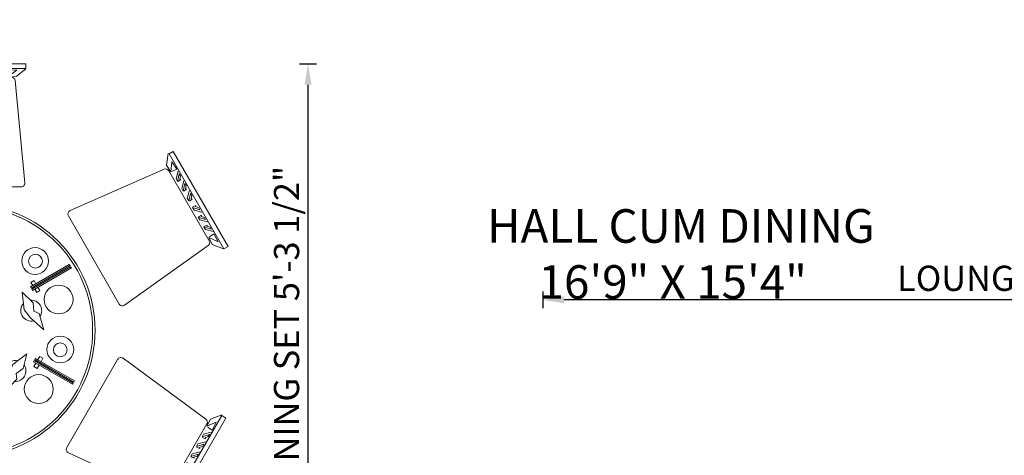
# Model space of a CAD drawing. Units: inches. Extents: x 1961 to 3038, y 800 to 1438.
# Tile 9 of 13: x 2803 to 2920, y 1096 to 1148. Entities that reach past the tile are written whole.
import ezdxf

# ---------------------------------------------------------------- set-up
doc = ezdxf.new("R2010")
doc.units = ezdxf.units.IN
for name, color, linetype, lineweight in [('A-ANNO-DIMS', 2, 'Continuous', 18), ('A-AREA-IDEN', 7, 'Continuous', 25), ('A-FURN', 8, 'Continuous', 18)]:
    doc.layers.add(name, color=color, linetype=linetype, lineweight=lineweight)
doc.styles.get("Standard").update_dxf_attribs({"font": 'arial.ttf'})
doc.dimstyles.new('ISO-25', dxfattribs={"dimtxt": 3, "dimasz": 2.5, "dimexe": 1, "dimexo": 1, "dimtad": 1, "dimdec": 4, "dimlunit": 4, "dimtxsty": 'Standard', "dimcen": 2.5, "dimadec": 0, "dimazin": 0, "dimtfac": 1, "dimtdec": 4, "dimtmove": 0, "dimatfit": 3, "dimfxl": 1, "dimfxlon": 1, "dimarcsym": 0})

# ---------------------------------------------------------------- blocks, each defined once
blk = doc.blocks.new('A$C1C317F9A')
for p, q in [((0.8788, 2.2685), (0.8788, 2.2478)), ((1.3449, 2.2685), (0.8788, 2.2685)), ((1.3449, 2.2478), (1.3449, 2.2685)), ((0.8756, 2.2462), (0.9155, 2.2143)), ((0.8788, 2.2478), (1.3449, 2.2478)), ((0.9139, 2.2414), (0.9522, 2.243)), ((0.949, 2.2159), (0.9139, 2.2414)), ((0.9522, 2.243), (0.9506, 2.2206)), ((0.9618, 2.2446), (0.9857, 2.2206)), ((0.9745, 2.243), (0.9841, 2.243)), ((0.9985, 2.2206), (0.9745, 2.243)), ((0.9841, 2.243), (0.9953, 2.2334)), ((0.9857, 2.2206), (0.9985, 2.2206)), ((0.9953, 2.2334), (0.9985, 2.2366)), ((0.9985, 2.2366), (1.0001, 2.2222)), ((1.0097, 2.2446), (1.0336, 2.2206)), ((1.0224, 2.243), (1.032, 2.243)), ((1.0464, 2.2206), (1.0224, 2.243)), ((1.032, 2.243), (1.0432, 2.2334)), ((1.0336, 2.2206), (1.0464, 2.2206)), ((1.0432, 2.2334), (1.0464, 2.2366)), ((1.0464, 2.2366), (1.048, 2.2222)), ((1.0576, 2.2446), (1.0815, 2.2206)), ((1.0703, 2.243), (1.0799, 2.243)), ((1.0943, 2.2206), (1.0703, 2.243)), ((1.0799, 2.243), (1.0911, 2.2334)), ((1.0815, 2.2206), (1.0943, 2.2206)), ((1.0911, 2.2334), (1.0943, 2.2366)), ((1.0943, 2.2366), (1.0959, 2.2222)), ((1.1262, 2.2366), (1.1246, 2.2222)), ((1.1262, 2.2206), (1.1502, 2.243)), ((1.1294, 2.2334), (1.1262, 2.2366)), ((1.139, 2.2206), (1.1262, 2.2206)), ((1.1406, 2.243), (1.1294, 2.2334)), ((1.1629, 2.2446), (1.139, 2.2206)), ((1.1502, 2.243), (1.1406, 2.243)), ((1.1741, 2.2366), (1.1725, 2.2222)), ((1.1741, 2.2206), (1.1981, 2.243)), ((1.1773, 2.2334), (1.1741, 2.2366)), ((1.1869, 2.2206), (1.1741, 2.2206)), ((1.1885, 2.243), (1.1773, 2.2334)), ((1.2108, 2.2446), (1.1869, 2.2206)), ((1.1981, 2.243), (1.1885, 2.243)), ((1.222, 2.2366), (1.2204, 2.2222)), ((1.222, 2.2206), (1.246, 2.243)), ((1.2252, 2.2334), (1.222, 2.2366)), ((1.2348, 2.2206), (1.222, 2.2206)), ((1.2364, 2.243), (1.2252, 2.2334)), ((1.2587, 2.2446), (1.2348, 2.2206)), ((1.246, 2.243), (1.2364, 2.243)), ((1.2683, 2.243), (1.2699, 2.2206)), ((1.3066, 2.2414), (1.2683, 2.243)), ((1.2715, 2.2159), (1.3066, 2.2414)), ((1.3449, 2.2462), (1.305, 2.2143)), ((0.8775, 1.7628), (0.9251, 2.1968)), ((0.9155, 2.2143), (0.949, 2.2159)), ((0.941, 2.2111), (1.2841, 2.2111)), ((1.305, 2.2143), (1.2715, 2.2159)), ((1.3, 2.1966), (1.3417, 1.7626)), ((0.2422, 1.9115), (0.0091, 1.5078)), ((0.0271, 1.4974), (0.2602, 1.9011)), ((0.2602, 1.9011), (0.2422, 1.9115)), ((0.2615, 1.9003), (0.2692, 1.8498)), ((1.9514, 1.8873), (1.9438, 1.8368)), ((1.9724, 1.8957), (1.9544, 1.8854)), ((1.9544, 1.8854), (2.1875, 1.4816)), ((2.2055, 1.492), (1.9724, 1.8957)), ((0.2465, 1.8648), (0.226, 1.8324)), ((0.2511, 1.8216), (0.2465, 1.8648)), ((0.2692, 1.8498), (0.2511, 1.8216)), ((1.9619, 1.8086), (1.9665, 1.8518)), ((1.9665, 1.8518), (1.987, 1.8194)), ((0.09, 1.5329), (0.2615, 1.8301)), ((0.2148, 1.813), (0.21, 1.8047)), ((0.21, 1.8047), (0.2127, 1.7903)), ((0.2222, 1.7811), (0.2148, 1.813)), ((0.2198, 1.8249), (0.2286, 1.7922)), ((0.226, 1.8324), (0.2461, 1.8226)), ((0.282, 1.8367), (0.6787, 1.6557)), ((1.5338, 1.644), (1.9335, 1.8198)), ((1.9438, 1.8368), (1.9619, 1.8086)), ((1.9537, 1.8131), (2.1253, 1.516)), ((1.987, 1.8194), (1.9669, 1.8096)), ((1.9932, 1.8119), (1.9844, 1.7792)), ((0.1909, 1.7716), (0.1861, 1.7633)), ((0.1861, 1.7633), (0.1888, 1.7488)), ((0.1982, 1.7396), (0.1909, 1.7716)), ((0.1959, 1.7834), (0.2046, 1.7507)), ((0.2127, 1.7903), (0.2084, 1.7891)), ((0.2084, 1.7891), (0.22, 1.7805)), ((0.2286, 1.7922), (0.2222, 1.7811)), ((1.9844, 1.7792), (1.9908, 1.7681)), ((1.9908, 1.7681), (1.9982, 1.8)), ((2.0046, 1.7761), (1.993, 1.7675)), ((1.9982, 1.8), (2.003, 1.7917)), ((2.003, 1.7917), (2.0003, 1.7773)), ((2.0003, 1.7773), (2.0046, 1.7761)), ((2.0171, 1.7704), (2.0084, 1.7377)), ((0.1669, 1.7301), (0.1621, 1.7218)), ((0.1621, 1.7218), (0.1648, 1.7073)), ((0.1743, 1.6982), (0.1669, 1.7301)), ((0.1719, 1.7419), (0.1807, 1.7092)), ((0.1888, 1.7488), (0.1844, 1.7476)), ((0.1844, 1.7476), (0.1961, 1.7391)), ((0.2046, 1.7507), (0.1982, 1.7396)), ((1.3258, 1.7451), (0.8934, 1.7451)), ((2.0084, 1.7377), (2.0147, 1.7266)), ((2.0147, 1.7266), (2.0221, 1.7585)), ((2.0286, 1.7346), (2.0169, 1.726)), ((2.0221, 1.7585), (2.0269, 1.7502)), ((2.0269, 1.7502), (2.0242, 1.7358)), ((2.0242, 1.7358), (2.0286, 1.7346)), ((2.0411, 1.7289), (2.0323, 1.6962)), ((2.0387, 1.6852), (2.0461, 1.7171)), ((2.0461, 1.7171), (2.0509, 1.7088)), ((0.1445, 1.6785), (0.1577, 1.6727)), ((0.1457, 1.6741), (0.1445, 1.6785)), ((0.1648, 1.7073), (0.1605, 1.7061)), ((0.1605, 1.7061), (0.1721, 1.6976)), ((0.1807, 1.7092), (0.1743, 1.6982)), ((2.0323, 1.6962), (2.0387, 1.6852)), ((2.0525, 1.6931), (2.0409, 1.6846)), ((2.0509, 1.7088), (2.0482, 1.6943)), ((2.0482, 1.6943), (2.0525, 1.6931)), ((0.1192, 1.6507), (0.1519, 1.6595)), ((0.1217, 1.6327), (0.1206, 1.637)), ((0.1206, 1.637), (0.1338, 1.6312)), ((0.1583, 1.6705), (0.127, 1.6609)), ((0.127, 1.6609), (0.1318, 1.6692)), ((0.1318, 1.6692), (0.1457, 1.6741)), ((0.1519, 1.6595), (0.1583, 1.6705)), ((0.6859, 1.6332), (0.4697, 1.2588)), ((1.091, 1.6437, 0.0908), (1.091, 1.4528, 0.0908)), ((1.097, 1.6437, 0.0908), (1.091, 1.6437, 0.0908)), ((1.097, 1.4528, 0.0908), (1.097, 1.6437, 0.0908)), ((1.1023, 1.6437, 0.0908), (1.1023, 1.4528, 0.0908)), ((1.1083, 1.6437, 0.0908), (1.1023, 1.6437, 0.0908)), ((1.1083, 1.4528, 0.0908), (1.1083, 1.6437, 0.0908)), ((2.0547, 1.6575), (2.086, 1.6479)), ((2.061, 1.6464), (2.0547, 1.6575)), ((2.0685, 1.6655), (2.0552, 1.6597)), ((2.0937, 1.6377), (2.061, 1.6464)), ((2.0673, 1.6611), (2.0685, 1.6655)), ((2.0812, 1.6562), (2.0673, 1.6611)), ((2.086, 1.6479), (2.0812, 1.6562)), ((0.0839, 1.5863), (0.0978, 1.5912)), ((0.0953, 1.6092), (0.128, 1.618)), ((0.0966, 1.5955), (0.1098, 1.5897)), ((0.0978, 1.5912), (0.0966, 1.5955)), ((0.1344, 1.629), (0.1031, 1.6195)), ((0.1031, 1.6195), (0.1078, 1.6278)), ((0.1078, 1.6278), (0.1217, 1.6327)), ((0.128, 1.618), (0.1344, 1.629)), ((1.7426, 1.2469), (1.5264, 1.6214)), ((2.0786, 1.616), (2.1099, 1.6065)), ((2.085, 1.605), (2.0786, 1.616)), ((2.0924, 1.624), (2.0792, 1.6182)), ((2.1177, 1.5962), (2.085, 1.605)), ((2.0913, 1.6196), (2.0924, 1.624)), ((2.1051, 1.6148), (2.0913, 1.6196)), ((2.1099, 1.6065), (2.1051, 1.6148)), ((0.0502, 1.5246), (0.0679, 1.5586)), ((0.0679, 1.5586), (0.0865, 1.5461)), ((0.0713, 1.5677), (0.104, 1.5765)), ((0.1104, 1.5876), (0.0791, 1.578)), ((0.0791, 1.578), (0.0839, 1.5863)), ((0.104, 1.5765), (0.1104, 1.5876)), ((2.1026, 1.5745), (2.1339, 1.565)), ((2.1089, 1.5635), (2.1026, 1.5745)), ((2.1164, 1.5825), (2.1031, 1.5767)), ((2.1416, 1.5547), (2.1089, 1.5635)), ((2.1152, 1.5782), (2.1164, 1.5825)), ((2.1291, 1.5733), (2.1152, 1.5782)), ((2.1339, 1.565), (2.1291, 1.5733)), ((0.0091, 1.5078), (0.0271, 1.4974)), ((0.0269, 1.4939), (0.0745, 1.5125)), ((0.0898, 1.5423), (0.0502, 1.5246)), ((0.0745, 1.5125), (0.0898, 1.5423)), ((0.4464, 1.2539), (0.0943, 1.5121)), ((2.1232, 1.5293), (2.1628, 1.5116)), ((2.1385, 1.4995), (2.1232, 1.5293)), ((2.145, 1.5456), (2.1265, 1.5331)), ((2.1628, 1.5116), (2.145, 1.5456)), ((1.0755, 1.4796, 0.0908), (1.0755, 1.4641, 0.0908)), ((1.091, 1.4796, 0.0908), (1.0755, 1.4796, 0.0908)), ((1.1023, 1.4796, 0.0908), (1.097, 1.4796, 0.0908)), ((1.125, 1.4796, 0.0908), (1.1083, 1.4796, 0.0908)), ((1.125, 1.4641, 0.0908), (1.125, 1.4796, 0.0908)), ((2.1208, 1.495), (1.7657, 1.2419)), ((2.1861, 1.4809), (2.1385, 1.4995)), ((2.1875, 1.4816), (2.2055, 1.492)), ((1.0755, 1.4641, 0.0908), (1.091, 1.4641, 0.0908)), ((1.091, 1.4528, 0.0908), (1.097, 1.4528, 0.0908)), ((1.1549, 1.429, 0.0908), (1.0933, 1.4112, 0.0908)), ((1.097, 1.4641, 0.0908), (1.1023, 1.4641, 0.0908)), ((1.1023, 1.4528, 0.0908), (1.1083, 1.4528, 0.0908)), ((1.1083, 1.4641, 0.0908), (1.125, 1.4641, 0.0908)), ((1.1882, 1.4134, 0.0908), (1.1549, 1.429, 0.0908)), ((1.2075, 1.4282, 0.0908), (1.1882, 1.4134, 0.0908)), ((1.278, 1.4112, 0.0908), (1.2075, 1.4282, 0.0908)), ((0.6765, 1.3825, 0.0908), (0.6735, 1.3774, 0.0908)), ((0.8419, 1.2871, 0.0908), (0.6765, 1.3825, 0.0908)), ((0.6822, 1.3924, 0.0908), (0.6792, 1.3872, 0.0908)), ((0.6792, 1.3872, 0.0908), (0.8446, 1.2917, 0.0908)), ((0.8476, 1.2969, 0.0908), (0.6822, 1.3924, 0.0908)), ((0.9684, 1.4231, 0.0908), (0.9184, 1.3706, 0.0908)), ((0.953, 1.3489, 0.0908), (0.9684, 1.4231, 0.0908)), ((1.0933, 1.4112, 0.0908), (1.1623, 1.3815, 0.0908)), ((1.1623, 1.3815, 0.0908), (1.2061, 1.3874, 0.0908)), ((1.2061, 1.3874, 0.0908), (1.278, 1.4112, 0.0908)), ((1.5304, 1.4154, 0.0908), (1.365, 1.3199, 0.0908)), ((1.368, 1.3147, 0.0908), (1.5334, 1.4102, 0.0908)), ((1.5361, 1.4055, 0.0908), (1.3707, 1.3101, 0.0908)), ((1.3737, 1.3049, 0.0908), (1.539, 1.4004, 0.0908)), ((1.5334, 1.4102, 0.0908), (1.5304, 1.4154, 0.0908)), ((1.539, 1.4004, 0.0908), (1.5361, 1.4055, 0.0908)), ((0.6735, 1.3774, 0.0908), (0.8389, 1.2819, 0.0908)), ((0.9216, 1.3464, 0.0908), (0.8914, 1.3253, 0.0908)), ((0.9184, 1.3706, 0.0908), (0.9216, 1.3464, 0.0908)), ((0.9363, 1.308, 0.0908), (0.953, 1.3489, 0.0908)), ((1.3805, 1.3467, 0.0908), (1.3671, 1.339, 0.0908)), ((1.3883, 1.3333, 0.0908), (1.3805, 1.3467, 0.0908)), ((0.8213, 1.3051, 0.0908), (0.8186, 1.3005, 0.0908)), ((0.8327, 1.3248, 0.0908), (0.8243, 1.3103, 0.0908)), ((0.8461, 1.317, 0.0908), (0.8327, 1.3248, 0.0908)), ((0.8377, 1.3025, 0.0908), (0.8461, 1.317, 0.0908)), ((0.8914, 1.3253, 0.0908), (0.8761, 1.2631, 0.0908)), ((0.8761, 1.2631, 0.0908), (0.9363, 1.308, 0.0908)), ((1.365, 1.3199, 0.0908), (1.368, 1.3147, 0.0908)), ((1.3671, 1.339, 0.0908), (1.3748, 1.3255, 0.0908)), ((1.3707, 1.3101, 0.0908), (1.3737, 1.3049, 0.0908)), ((1.3778, 1.3204, 0.0908), (1.3805, 1.3157, 0.0908)), ((1.3835, 1.3106, 0.0908), (1.3918, 1.2961, 0.0908)), ((1.3939, 1.3235, 0.0908), (1.3912, 1.3281, 0.0908)), ((1.3918, 1.2961, 0.0908), (1.4053, 1.3038, 0.0908)), ((1.4053, 1.3038, 0.0908), (1.3969, 1.3183, 0.0908)), ((0.8156, 1.2953, 0.0908), (0.8079, 1.2819, 0.0908)), ((0.8079, 1.2819, 0.0908), (0.8213, 1.2741, 0.0908)), ((0.8213, 1.2741, 0.0908), (0.8291, 1.2876, 0.0908)), ((0.8321, 1.2927, 0.0908), (0.8348, 1.2974, 0.0908)), ((0.8389, 1.2819, 0.0908), (0.8419, 1.2871, 0.0908)), ((0.8446, 1.2917, 0.0908), (0.8476, 1.2969, 0.0908)), ((1.3763, 1.2527, 0.0908), (1.3301, 1.2971, 0.0908)), ((1.3301, 1.2971, 0.0908), (1.3389, 1.2225, 0.0908)), ((1.3389, 1.2225, 0.0908), (1.366, 1.1876, 0.0908)), ((1.3795, 1.216, 0.0908), (1.3763, 1.2527, 0.0908)), ((1.402, 1.2067, 0.0908), (1.3795, 1.216, 0.0908)), ((1.366, 1.1876, 0.0908), (1.4225, 1.1371, 0.0908)), ((1.4225, 1.1371, 0.0908), (1.402, 1.2067, 0.0908)), ((0.8033, 1.1609, 0.0908), (0.8238, 1.0913, 0.0908)), ((0.8599, 1.1105, 0.0908), (0.8033, 1.1609, 0.0908)), ((0.8238, 1.0913, 0.0908), (0.8463, 1.0821, 0.0908)), ((0.8869, 1.0755, 0.0908), (0.8599, 1.1105, 0.0908)), ((0.8463, 1.0821, 0.0908), (0.8495, 1.0454, 0.0908)), ((0.8957, 1.0009, 0.0908), (0.8869, 1.0755, 0.0908)), ((0.0847, 0.7751), (0.4398, 1.0281)), ((0.4628, 1.0231), (0.679, 0.6486)), ((0.8495, 1.0454, 0.0908), (0.8957, 1.0009, 0.0908)), ((1.3498, 1.0349, 0.0908), (1.2896, 0.99, 0.0908)), ((1.3344, 0.9727, 0.0908), (1.3498, 1.0349, 0.0908)), ((1.3813, 1.0063, 0.0908), (1.3783, 1.0011, 0.0908)), ((1.5466, 0.9108, 0.0908), (1.3813, 1.0063, 0.0908)), ((1.3869, 1.0161, 0.0908), (1.384, 1.011, 0.0908)), ((1.384, 1.011, 0.0908), (1.5493, 0.9155, 0.0908)), ((1.5523, 0.9207, 0.0908), (1.3869, 1.0161, 0.0908)), ((1.3938, 1.0053, 0.0908), (1.3911, 1.0006, 0.0908)), ((1.4045, 1.0239, 0.0908), (1.3968, 1.0105, 0.0908)), ((1.418, 1.0162, 0.0908), (1.4045, 1.0239, 0.0908)), ((1.4102, 1.0027, 0.0908), (1.418, 1.0162, 0.0908)), ((1.5196, 0.6368), (1.7358, 1.0113)), ((1.7591, 1.0162), (2.1111, 0.7579)), ((0.8522, 0.9931, 0.0908), (0.6868, 0.8977, 0.0908)), ((0.6898, 0.8925, 0.0908), (0.8552, 0.988, 0.0908)), ((0.8578, 0.9833, 0.0908), (0.6925, 0.8878, 0.0908)), ((0.6955, 0.8827, 0.0908), (0.8608, 0.9781, 0.0908)), ((0.834, 1.0019, 0.0908), (0.8206, 0.9942, 0.0908)), ((0.8206, 0.9942, 0.0908), (0.8289, 0.9797, 0.0908)), ((0.8319, 0.9745, 0.0908), (0.8346, 0.9699, 0.0908)), ((0.8424, 0.9875, 0.0908), (0.834, 1.0019, 0.0908)), ((0.8376, 0.9647, 0.0908), (0.8453, 0.9513, 0.0908)), ((0.848, 0.9776, 0.0908), (0.8453, 0.9823, 0.0908)), ((0.8588, 0.959, 0.0908), (0.851, 0.9725, 0.0908)), ((0.8552, 0.988, 0.0908), (0.8522, 0.9931, 0.0908)), ((0.8608, 0.9781, 0.0908), (0.8578, 0.9833, 0.0908)), ((1.2896, 0.99, 0.0908), (1.2728, 0.9491, 0.0908)), ((1.3042, 0.9516, 0.0908), (1.3344, 0.9727, 0.0908)), ((1.3783, 1.0011, 0.0908), (1.5437, 0.9057, 0.0908)), ((1.3881, 0.9955, 0.0908), (1.3797, 0.981, 0.0908)), ((1.3797, 0.981, 0.0908), (1.3932, 0.9732, 0.0908)), ((1.3932, 0.9732, 0.0908), (1.4015, 0.9877, 0.0908)), ((1.4045, 0.9929, 0.0908), (1.4072, 0.9975, 0.0908)), ((0.8453, 0.9513, 0.0908), (0.8588, 0.959, 0.0908)), ((1.2728, 0.9491, 0.0908), (1.2574, 0.875, 0.0908)), ((1.2574, 0.875, 0.0908), (1.3074, 0.9275, 0.0908)), ((1.3074, 0.9275, 0.0908), (1.3042, 0.9516, 0.0908)), ((0.6868, 0.8977, 0.0908), (0.6898, 0.8925, 0.0908)), ((0.6925, 0.8878, 0.0908), (0.6955, 0.8827, 0.0908)), ((1.0198, 0.9106, 0.0908), (0.9478, 0.8869, 0.0908)), ((0.9478, 0.8869, 0.0908), (1.0183, 0.8698, 0.0908)), ((1.0183, 0.8698, 0.0908), (1.0376, 0.8846, 0.0908)), ((1.0636, 0.9165, 0.0908), (1.0198, 0.9106, 0.0908)), ((1.0376, 0.8846, 0.0908), (1.071, 0.8691, 0.0908)), ((1.1326, 0.8869, 0.0908), (1.0636, 0.9165, 0.0908)), ((1.071, 0.8691, 0.0908), (1.1326, 0.8869, 0.0908)), ((1.5437, 0.9057, 0.0908), (1.5466, 0.9108, 0.0908)), ((1.5493, 0.9155, 0.0908), (1.5523, 0.9207, 0.0908)), ((1.1235, 0.8453, 0.0908), (1.1175, 0.8453, 0.0908)), ((1.1175, 0.8453, 0.0908), (1.1175, 0.6543, 0.0908)), ((1.1235, 0.6543, 0.0908), (1.1235, 0.8453, 0.0908)), ((1.1349, 0.8453, 0.0908), (1.1289, 0.8453, 0.0908)), ((1.1289, 0.8453, 0.0908), (1.1289, 0.6543, 0.0908)), ((1.1349, 0.6543, 0.0908), (1.1349, 0.8453, 0.0908)), ((1.1175, 0.8339, 0.0908), (1.1008, 0.8339, 0.0908)), ((1.1008, 0.8339, 0.0908), (1.1008, 0.8184, 0.0908)), ((1.1008, 0.8184, 0.0908), (1.1175, 0.8184, 0.0908)), ((1.1289, 0.8339, 0.0908), (1.1235, 0.8339, 0.0908)), ((1.1235, 0.8184, 0.0908), (1.1289, 0.8184, 0.0908)), ((1.1504, 0.8339, 0.0908), (1.1349, 0.8339, 0.0908)), ((1.1349, 0.8184, 0.0908), (1.1504, 0.8184, 0.0908)), ((1.1504, 0.8184, 0.0908), (1.1504, 0.8339, 0.0908)), ((0.018, 0.7884), (0, 0.778)), ((0, 0.778), (0.2331, 0.3743)), ((0.2511, 0.3847), (0.018, 0.7884)), ((0.0193, 0.7892), (0.0669, 0.7706)), ((0.0427, 0.7584), (0.0604, 0.7244)), ((0.0823, 0.7407), (0.0427, 0.7584)), ((0.0669, 0.7706), (0.0823, 0.7407)), ((0.2517, 0.4569), (0.0802, 0.7541)), ((2.1784, 0.7726), (1.9453, 0.3689)), ((1.9633, 0.3585), (2.1964, 0.7622)), ((2.131, 0.7576), (2.1156, 0.7277)), ((2.1786, 0.7762), (2.131, 0.7576)), ((2.1964, 0.7622), (2.1784, 0.7726)), ((0.0604, 0.7244), (0.079, 0.737)), ((0.0638, 0.7153), (0.0965, 0.7066)), ((2.1155, 0.7371), (1.9439, 0.4399)), ((2.1156, 0.7277), (2.1553, 0.7454)), ((2.1375, 0.7114), (2.119, 0.724)), ((2.1553, 0.7454), (2.1375, 0.7114)), ((0.0716, 0.7051), (0.0764, 0.6968)), ((0.1029, 0.6955), (0.0716, 0.7051)), ((0.0764, 0.6968), (0.0903, 0.6919)), ((0.0878, 0.6738), (0.1205, 0.6651)), ((0.0891, 0.6875), (0.1023, 0.6933)), ((0.0903, 0.6919), (0.0891, 0.6875)), ((0.0965, 0.7066), (0.1029, 0.6955)), ((2.1014, 0.6935), (2.095, 0.6825)), ((2.095, 0.6825), (2.1264, 0.6921)), ((2.1089, 0.6745), (2.0956, 0.6803)), ((2.1341, 0.7023), (2.1014, 0.6935)), ((2.1216, 0.6838), (2.1077, 0.6789)), ((2.1077, 0.6789), (2.1089, 0.6745)), ((2.1264, 0.6921), (2.1216, 0.6838)), ((0.0955, 0.6636), (0.1003, 0.6553)), ((0.1269, 0.654), (0.0955, 0.6636)), ((0.1003, 0.6553), (0.1142, 0.6504)), ((0.1117, 0.6324), (0.1444, 0.6236)), ((0.1131, 0.646), (0.1263, 0.6518)), ((0.1142, 0.6504), (0.1131, 0.646)), ((0.1205, 0.6651), (0.1269, 0.654)), ((1.1175, 0.6543, 0.0908), (1.1235, 0.6543, 0.0908)), ((1.1289, 0.6543, 0.0908), (1.1349, 0.6543, 0.0908)), ((2.0775, 0.6521), (2.0711, 0.641)), ((2.0711, 0.641), (2.1024, 0.6506)), ((2.0849, 0.633), (2.0717, 0.6388)), ((2.1102, 0.6608), (2.0775, 0.6521)), ((2.0976, 0.6423), (2.0837, 0.6374)), ((2.0837, 0.6374), (2.0849, 0.633)), ((2.1024, 0.6506), (2.0976, 0.6423)), ((0.1195, 0.6221), (0.1243, 0.6138)), ((0.1508, 0.6125), (0.1195, 0.6221)), ((0.1243, 0.6138), (0.1382, 0.6089)), ((0.137, 0.6046), (0.1502, 0.6104)), ((0.1382, 0.6089), (0.137, 0.6046)), ((0.1444, 0.6236), (0.1508, 0.6125)), ((0.6716, 0.6261), (0.272, 0.4503)), ((1.9235, 0.4334), (1.5268, 0.6143)), ((2.0535, 0.6106), (2.0471, 0.5995)), ((2.0471, 0.5995), (2.0785, 0.6091)), ((2.061, 0.5915), (2.0477, 0.5973)), ((2.0862, 0.6194), (2.0535, 0.6106)), ((2.0737, 0.6008), (2.0598, 0.5959)), ((2.0598, 0.5959), (2.061, 0.5915)), ((2.0785, 0.6091), (2.0737, 0.6008)), ((0.153, 0.5769), (0.1646, 0.5855)), ((0.1573, 0.5757), (0.153, 0.5769)), ((0.1546, 0.5613), (0.1573, 0.5757)), ((0.1594, 0.553), (0.1546, 0.5613)), ((0.1668, 0.5849), (0.1594, 0.553)), ((0.1644, 0.5411), (0.1732, 0.5738)), ((0.1732, 0.5738), (0.1668, 0.5849)), ((2.0248, 0.5608), (2.0312, 0.5719)), ((2.0336, 0.5281), (2.0248, 0.5608)), ((2.0312, 0.5719), (2.0386, 0.54)), ((2.045, 0.5639), (2.0334, 0.5725)), ((2.0386, 0.54), (2.0433, 0.5483)), ((2.0406, 0.5627), (2.045, 0.5639)), ((2.0433, 0.5483), (2.0406, 0.5627)), ((0.1769, 0.5354), (0.1885, 0.544)), ((0.1813, 0.5343), (0.1769, 0.5354)), ((0.1786, 0.5198), (0.1813, 0.5343)), ((0.1834, 0.5115), (0.1786, 0.5198)), ((0.1907, 0.5434), (0.1834, 0.5115)), ((0.1884, 0.4996), (0.1971, 0.5323)), ((0.1971, 0.5323), (0.1907, 0.5434)), ((0.2009, 0.4939), (0.2125, 0.5025)), ((0.9055, 0.0734), (0.8638, 0.5074)), ((0.9096, 0.0719), (0.8679, 0.5059)), ((0.8797, 0.5249), (1.3121, 0.5249)), ((0.8838, 0.5234), (1.3162, 0.5234)), ((1.328, 0.5072), (1.2804, 0.0732)), ((1.3321, 0.5057), (1.2845, 0.0717)), ((2.0009, 0.5193), (2.0072, 0.5304)), ((2.0096, 0.4866), (2.0009, 0.5193)), ((2.0072, 0.5304), (2.0146, 0.4985)), ((2.0211, 0.5224), (2.0094, 0.531)), ((2.0146, 0.4985), (2.0194, 0.5068)), ((2.0167, 0.5212), (2.0211, 0.5224)), ((2.0194, 0.5068), (2.0167, 0.5212)), ((0.2052, 0.4928), (0.2009, 0.4939)), ((0.2025, 0.4783), (0.2052, 0.4928)), ((0.2073, 0.47), (0.2025, 0.4783)), ((0.2147, 0.5019), (0.2073, 0.47)), ((0.2123, 0.4582), (0.2211, 0.4909)), ((0.2211, 0.4909), (0.2147, 0.5019)), ((0.2436, 0.4615), (0.239, 0.4183)), ((0.2617, 0.4332), (0.2436, 0.4615)), ((1.9769, 0.4779), (1.9833, 0.4889)), ((1.9857, 0.4451), (1.9769, 0.4779)), ((1.9833, 0.4889), (1.9907, 0.457)), ((1.9971, 0.4809), (1.9855, 0.4895)), ((1.9907, 0.457), (1.9955, 0.4653)), ((1.9927, 0.4798), (1.9971, 0.4809)), ((1.9955, 0.4653), (1.9927, 0.4798)), ((0.2185, 0.4507), (0.2386, 0.4604)), ((0.239, 0.4183), (0.2185, 0.4507)), ((0.254, 0.3827), (0.2617, 0.4332)), ((1.9363, 0.4202), (1.9544, 0.4484)), ((1.9439, 0.3697), (1.9363, 0.4202)), ((1.9544, 0.4484), (1.9589, 0.4053)), ((1.9589, 0.4053), (1.9795, 0.4377)), ((1.9795, 0.4377), (1.9593, 0.4474)), ((0.2331, 0.3743), (0.2511, 0.3847)), ((1.9453, 0.3689), (1.9633, 0.3585)), ((0.8605, 0.0239), (0.9005, 0.0558)), ((0.8647, 0.0223), (0.9046, 0.0543)), ((0.934, 0.0542), (0.8989, 0.0286)), ((0.9005, 0.0558), (0.934, 0.0542)), ((0.9381, 0.0527), (0.903, 0.0271)), ((0.9046, 0.0543), (0.9381, 0.0527)), ((1.2645, 0.059), (0.9213, 0.059)), ((1.2686, 0.0574), (0.9255, 0.0574)), ((0.9372, 0.027), (0.9356, 0.0494)), ((0.9413, 0.0255), (0.9397, 0.0479)), ((0.9468, 0.0255), (0.9707, 0.0494)), ((0.9509, 0.0239), (0.9748, 0.0479)), ((0.9835, 0.0494), (0.9595, 0.027)), ((0.9876, 0.0479), (0.9636, 0.0255)), ((0.9707, 0.0494), (0.9835, 0.0494)), ((0.9748, 0.0479), (0.9876, 0.0479)), ((0.9835, 0.0334), (0.9851, 0.0478)), ((0.9876, 0.0319), (0.9892, 0.0463)), ((0.9946, 0.0255), (1.0186, 0.0494)), ((0.9988, 0.0239), (1.0227, 0.0479)), ((1.0314, 0.0494), (1.0074, 0.027)), ((1.0355, 0.0479), (1.0115, 0.0255)), ((1.0186, 0.0494), (1.0314, 0.0494)), ((1.0227, 0.0479), (1.0355, 0.0479)), ((1.0314, 0.0334), (1.033, 0.0478)), ((1.0355, 0.0319), (1.0371, 0.0463)), ((1.0425, 0.0255), (1.0665, 0.0494)), ((1.0467, 0.0239), (1.0706, 0.0479)), ((1.0793, 0.0494), (1.0553, 0.027)), ((1.0834, 0.0479), (1.0594, 0.0255)), ((1.0665, 0.0494), (1.0793, 0.0494)), ((1.0706, 0.0479), (1.0834, 0.0479)), ((1.0793, 0.0334), (1.0809, 0.0478)), ((1.0834, 0.0319), (1.085, 0.0463)), ((1.1112, 0.0334), (1.1096, 0.0478)), ((1.1112, 0.0494), (1.1351, 0.027)), ((1.124, 0.0494), (1.1112, 0.0494)), ((1.1153, 0.0319), (1.1137, 0.0463)), ((1.1153, 0.0479), (1.1393, 0.0255)), ((1.1281, 0.0479), (1.1153, 0.0479)), ((1.1479, 0.0255), (1.124, 0.0494)), ((1.152, 0.0239), (1.1281, 0.0479)), ((1.1591, 0.0334), (1.1575, 0.0478)), ((1.1591, 0.0494), (1.183, 0.027)), ((1.1719, 0.0494), (1.1591, 0.0494)), ((1.1632, 0.0319), (1.1616, 0.0463)), ((1.1632, 0.0479), (1.1872, 0.0255)), ((1.176, 0.0479), (1.1632, 0.0479)), ((1.1958, 0.0255), (1.1719, 0.0494)), ((1.1999, 0.0239), (1.176, 0.0479)), ((1.207, 0.0334), (1.2054, 0.0478)), ((1.207, 0.0494), (1.2309, 0.027)), ((1.2198, 0.0494), (1.207, 0.0494)), ((1.2111, 0.0319), (1.2095, 0.0463)), ((1.2111, 0.0479), (1.235, 0.0255)), ((1.2239, 0.0479), (1.2111, 0.0479)), ((1.2437, 0.0255), (1.2198, 0.0494)), ((1.2478, 0.0239), (1.2239, 0.0479)), ((1.2533, 0.027), (1.2549, 0.0494)), ((1.29, 0.0558), (1.2565, 0.0542)), ((1.2565, 0.0542), (1.2916, 0.0286)), ((1.2574, 0.0255), (1.259, 0.0479)), ((1.2941, 0.0543), (1.2606, 0.0527)), ((1.2606, 0.0527), (1.2957, 0.0271)), ((1.3299, 0.0239), (1.29, 0.0558)), ((1.334, 0.0223), (1.2941, 0.0543)), ((0.8605, 0.0223), (0.8605, 0.0015)), ((1.3267, 0.0223), (0.8605, 0.0223)), ((0.8605, 0.0015), (1.3267, 0.0015)), ((0.8647, 0.0207), (0.8647, 0)), ((1.3308, 0.0207), (0.8647, 0.0207)), ((0.8647, 0), (1.3308, 0)), ((0.8989, 0.0286), (0.9372, 0.027)), ((0.903, 0.0271), (0.9413, 0.0255)), ((0.9595, 0.027), (0.9691, 0.027)), ((0.9636, 0.0255), (0.9732, 0.0255)), ((0.9691, 0.027), (0.9803, 0.0366)), ((0.9732, 0.0255), (0.9844, 0.0351)), ((0.9803, 0.0366), (0.9835, 0.0334)), ((0.9844, 0.0351), (0.9876, 0.0319)), ((1.0074, 0.027), (1.017, 0.027)), ((1.0115, 0.0255), (1.0211, 0.0255)), ((1.017, 0.027), (1.0282, 0.0366)), ((1.0211, 0.0255), (1.0323, 0.0351)), ((1.0282, 0.0366), (1.0314, 0.0334)), ((1.0323, 0.0351), (1.0355, 0.0319)), ((1.0553, 0.027), (1.0649, 0.027)), ((1.0594, 0.0255), (1.069, 0.0255)), ((1.0649, 0.027), (1.0761, 0.0366)), ((1.069, 0.0255), (1.0802, 0.0351)), ((1.0761, 0.0366), (1.0793, 0.0334)), ((1.0802, 0.0351), (1.0834, 0.0319)), ((1.1144, 0.0366), (1.1112, 0.0334)), ((1.1256, 0.027), (1.1144, 0.0366)), ((1.1185, 0.0351), (1.1153, 0.0319)), ((1.1297, 0.0255), (1.1185, 0.0351)), ((1.1351, 0.027), (1.1256, 0.027)), ((1.1393, 0.0255), (1.1297, 0.0255)), ((1.1623, 0.0366), (1.1591, 0.0334)), ((1.1735, 0.027), (1.1623, 0.0366)), ((1.1664, 0.0351), (1.1632, 0.0319)), ((1.1776, 0.0255), (1.1664, 0.0351)), ((1.183, 0.027), (1.1735, 0.027)), ((1.1872, 0.0255), (1.1776, 0.0255)), ((1.2102, 0.0366), (1.207, 0.0334)), ((1.2214, 0.027), (1.2102, 0.0366)), ((1.2143, 0.0351), (1.2111, 0.0319)), ((1.2255, 0.0255), (1.2143, 0.0351)), ((1.2309, 0.027), (1.2214, 0.027)), ((1.235, 0.0255), (1.2255, 0.0255)), ((1.2916, 0.0286), (1.2533, 0.027)), ((1.2957, 0.0271), (1.2574, 0.0255)), ((1.3267, 0.0015), (1.3267, 0.0223)), ((1.3308, 0), (1.3308, 0.0207))]:
    blk.add_line(p, q)
for centre, radius in [((1.1027, 1.135), 0.537), ((1.1027, 1.135), 0.527), ((1.0059, 1.525, 0.0908), 0.0569), ((1.0072, 1.5257, 0.0908), 0.0294), ((1.1975, 1.5297, 0.0908), 0.0613), ((0.8256, 1.4126, 0.0908), 0.0613), ((1.385, 1.4297, 0.0908), 0.0569), ((1.3863, 1.4289, 0.0908), 0.0294), ((0.7338, 1.2443, 0.0908), 0.0569), ((1.4849, 1.2661, 0.0908), 0.0613), ((0.7339, 1.2458, 0.0908), 0.0294), ((0.741, 1.0319, 0.0908), 0.0613), ((1.4921, 1.0537, 0.0908), 0.0569), ((1.492, 1.0522, 0.0908), 0.0294), ((0.8408, 0.8683, 0.0908), 0.0569), ((1.4003, 0.8854, 0.0908), 0.0613), ((0.8396, 0.8691, 0.0908), 0.0294), ((1.0283, 0.7683, 0.0908), 0.0613), ((1.2199, 0.773, 0.0908), 0.0569), ((1.2186, 0.7723, 0.0908), 0.0294)]:
    blk.add_circle(centre, radius)
for centre, radius, start, end in [((0.941, 2.1951), 0.016, 90, 173.7428), ((1.2841, 2.1951), 0.016, 5.4801, 90), ((0.2754, 1.8222), 0.016, 65.4801, 150), ((1.9399, 1.8052), 0.016, 30, 113.7428), ((0.8934, 1.7611), 0.016, 173.7428, 270), ((1.3258, 1.7611), 0.016, 270, 5.4801), ((0.6721, 1.6412), 0.016, 330, 65.4801), ((1.5403, 1.6294), 0.016, 113.7428, 210), ((0.1038, 1.525), 0.016, 150, 233.7428), ((2.1115, 1.508), 0.016, 305.4801, 30), ((1.1801, 1.4052, 0.0908), 0.0446, 26.6641, 154.1442), ((1.1801, 1.4052, 0.0908), 0.0446, 197.0611, 344.0662), ((0.9246, 1.3353, 0.0908), 0.0446, 86.6641, 214.1442), ((0.9246, 1.3353, 0.0908), 0.0446, 257.0611, 44.0662), ((0.4559, 1.2667), 0.016, 233.7428, 330), ((1.3684, 1.2189, 0.0908), 0.0446, 326.6641, 94.1442), ((1.3684, 1.2189, 0.0908), 0.0446, 137.0611, 284.0662), ((1.7565, 1.2549), 0.016, 210, 305.4801), ((0.8574, 1.0791, 0.0908), 0.0446, 146.6641, 274.1442), ((0.8574, 1.0791, 0.0908), 0.0446, 317.0611, 104.0662), ((0.449, 1.0151), 0.016, 30, 125.4801), ((1.3012, 0.9627, 0.0908), 0.0446, 77.0611, 224.0662), ((1.7496, 1.0033), 0.016, 53.7428, 150), ((1.3012, 0.9627, 0.0908), 0.0446, 266.6641, 34.1442), ((1.0457, 0.8928, 0.0908), 0.0446, 17.0611, 164.0662), ((1.0457, 0.8928, 0.0908), 0.0446, 206.6641, 334.1442), ((0.094, 0.7621), 0.016, 125.4801, 210), ((2.1017, 0.7451), 0.016, 330, 53.7428), ((0.6652, 0.6407), 0.016, 293.7428, 30), ((1.5334, 0.6288), 0.016, 150, 245.4801), ((0.8797, 0.5089), 0.016, 90, 185.4801), ((0.8838, 0.5074), 0.016, 90, 185.4801), ((1.3121, 0.5089), 0.016, 353.7428, 90), ((1.3162, 0.5074), 0.016, 353.7428, 90), ((0.2656, 0.4649), 0.016, 210, 293.7428), ((1.9301, 0.4479), 0.016, 245.4801, 330), ((0.9213, 0.0749), 0.016, 185.4801, 270), ((0.9255, 0.0734), 0.016, 185.4801, 270), ((1.2645, 0.0749), 0.016, 270, 353.7428), ((1.2686, 0.0734), 0.016, 270, 353.7428)]:
    blk.add_arc(centre, radius, start, end)
blk = doc.blocks.new('*D61')
at = {"layer": 'A-ANNO-DIMS', "color": 0, "lineweight": -2, "transparency": 16777216}
for p, q in [((2836.59, 1142.53), (2838.59, 1142.53)), ((2837.59, 1081.54), (2837.59, 1140.03)), ((2836.59, 1079.04), (2838.59, 1079.04))]:
    blk.add_line(p, q, dxfattribs=at)
at = {"layer": 'A-ANNO-DIMS', "color": 0, "transparency": 16777216}
for points in [[(2837.18, 1140.03), (2838.01, 1140.03), (2837.59, 1142.53)], [(2837.18, 1081.54), (2838.01, 1081.54), (2837.59, 1079.04)]]:
    blk.add_solid(points, dxfattribs=at)
at = {"layer": 'Defpoints', "color": 0, "transparency": 16777216}
for p in [(2828.07, 1142.53), (2837.59, 1142.53), (2828.07, 1079.04)]:
    blk.add_point(p, dxfattribs=at)
at = {"layer": 'A-ANNO-DIMS', "color": 0, "transparency": 16777216, "insert": (2835.42, 1110.79), "char_height": 3, "attachment_point": 5, "rotation": 90}
blk.add_mtext('DINING SET 5\'-3 1/2"', dxfattribs=at)
blk = doc.blocks.new('*D63')
at = {"layer": 'A-ANNO-DIMS', "color": 0, "lineweight": -2, "transparency": 16777216}
for p, q in [((2865.57, 1113.43), (2865.57, 1115.43)), ((2986.68, 1113.43), (2986.68, 1115.43)), ((2984.18, 1114.43), (2868.07, 1114.43))]:
    blk.add_line(p, q, dxfattribs=at)
at = {"layer": 'A-ANNO-DIMS', "color": 0, "transparency": 16777216}
for points in [[(2868.07, 1114.85), (2868.07, 1114.02), (2865.57, 1114.43)], [(2984.18, 1114.85), (2984.18, 1114.02), (2986.68, 1114.43)]]:
    blk.add_solid(points, dxfattribs=at)
at = {"layer": 'Defpoints', "color": 0, "transparency": 16777216}
for p in [(2865.57, 1114.43), (2865.57, 1096.27), (2986.68, 1096.27)]:
    blk.add_point(p, dxfattribs=at)
at = {"layer": 'A-ANNO-DIMS', "color": 0, "transparency": 16777216, "insert": (2926.13, 1116.61), "char_height": 3, "attachment_point": 5}
blk.add_mtext('LOUNGE SET 10\'-1"', dxfattribs=at)
blk = doc.blocks.new('*D75')
at = {"layer": 'A-ANNO-DIMS', "color": 0, "lineweight": -2, "transparency": 16777216}
for p, q in [((2809.27, 1340.52), (2809.27, 1342.52)), ((2845.27, 1340.52), (2845.27, 1342.52)), ((2811.77, 1341.52), (2842.77, 1341.52))]:
    blk.add_line(p, q, dxfattribs=at)
at = {"layer": 'A-ANNO-DIMS', "color": 0, "transparency": 16777216}
for points in [[(2811.77, 1341.94), (2811.77, 1341.1), (2809.27, 1341.52)], [(2842.77, 1341.94), (2842.77, 1341.1), (2845.27, 1341.52)]]:
    blk.add_solid(points, dxfattribs=at)
at = {"layer": 'Defpoints', "color": 0, "transparency": 16777216}
for p in [(2845.27, 1341.52), (2809.27, 970.92), (2845.27, 970.92)]:
    blk.add_point(p, dxfattribs=at)
at = {"layer": 'A-ANNO-DIMS', "color": 0, "transparency": 16777216, "insert": (2827.27, 1343.68), "char_height": 3, "attachment_point": 5}
blk.add_mtext('3\'-0"', dxfattribs=at)

msp = doc.modelspace()

# ---------------------------------------------------------------- block references
at = {"layer": 'A-FURN', "xscale": 27.98955775126368, "yscale": 27.98955775126368, "zscale": 27.98955775126368}
msp.add_blockref('A$C1C317F9A', (2766.339, 1079.03804, -2.54052), dxfattribs=at)

# ---------------------------------------------------------------- texts
at = {"layer": 'A-AREA-IDEN', "insert": (2858.91292, 1125.22542), "char_height": 4, "attachment_point": 1}
msp.add_mtext_dynamic_manual_height_columns('{\\fTimes New Roman|b1|i0|c0|p18;HALL CUM DINING\\P     16\'9" X 15\'4"}', width=58.2616082, gutter_width=12.5, heights=[0], dxfattribs=at)

# ---------------------------------------------------------------- dimensions: what is measured, and where the dimension line sits
at = {"layer": 'A-ANNO-DIMS'}
dim = msp.add_linear_dim(base=(2845.26803, 1341.51975), p1=(2809.26803, 970.91975), p2=(2845.26803, 970.91975), dimstyle='ISO-25', override={"dimdec": 1, "dimlfac": 1, "dimrnd": 0, "dimzin": 1, "dimdsep": 46, "dimlunit": 4, "dimfrac": 2}, dxfattribs=at)
dim.commit()
dim.dimension.update_dxf_attribs({"geometry": '*D75', "text_midpoint": (2827.26803, 1343.6775)})
for base, p1, p2, angle, text, picture, middle in [((2837.59352, 1142.53289), (2828.0693, 1079.03804), (2828.0693, 1142.53289), 90, 'DINING SET <>', '*D61', (2835.41634, 1110.78547)), ((2865.57325, 1114.43305), (2986.6849, 1096.26631), (2865.57325, 1096.26631), 180, 'LOUNGE SET <>', '*D63', (2926.12907, 1116.61024))]:
    dim = msp.add_linear_dim(base=base, p1=p1, p2=p2, angle=angle, text=text, dimstyle='ISO-25', override={"dimdec": 1, "dimlfac": 1, "dimrnd": 0, "dimzin": 1, "dimdsep": 46, "dimlunit": 4, "dimfrac": 2}, dxfattribs=at)
    dim.commit()
    dim.dimension.update_dxf_attribs({"geometry": picture, "text_midpoint": middle})

doc.saveas('drawing.dxf')
